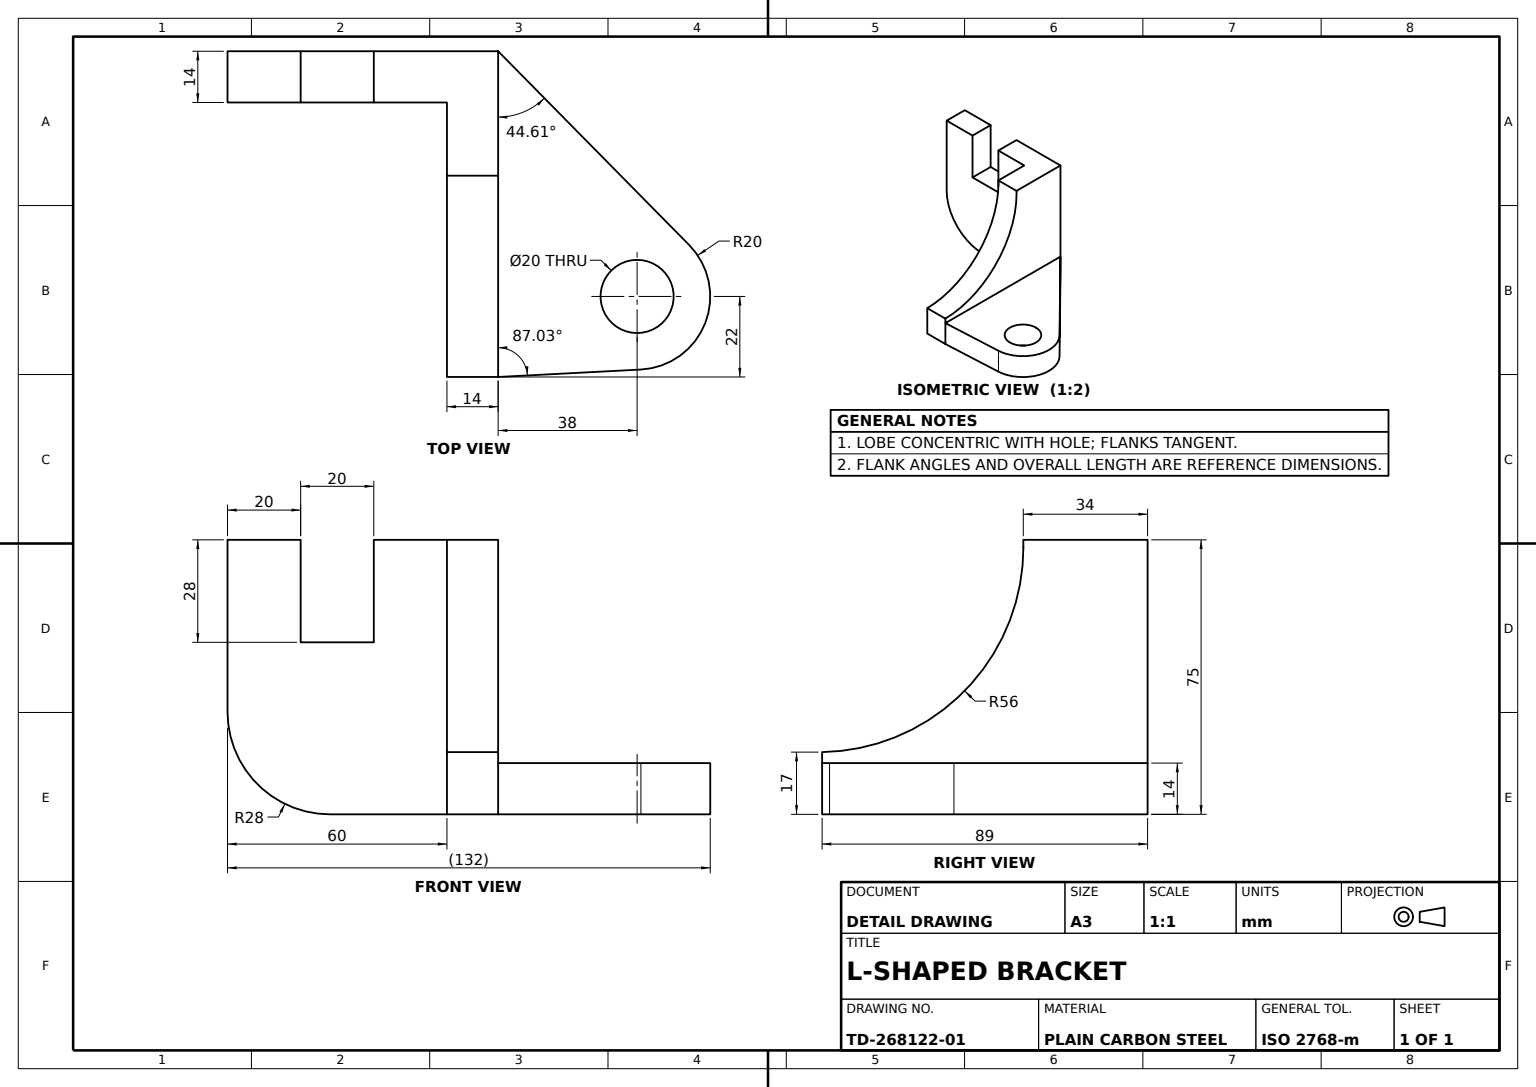
SolidWorks part; units mm, degrees
material "Plain Carbon Steel"
ref_plane "Front Plane" through (0, 0, 0) normal (0, 0, 1) x (1, 0, 0)
ref_plane "Top Plane" through (0, 0, 0) normal (0, 1, 0) x (1, 0, 0)
ref_plane "Right Plane" through (0, 0, 0) normal (1, 0, 0) x (0, 0, -1)
sketch "Base Plate Profile" plane through (0, 0, 0) normal (0, 0, 1) x (1, 0, 0)
  line L0 (0, 0) -> (0, 75)
  line L1 (0, 75) -> (32, 75)
  line L2 (60, 47) -> (60, 0)
  line L3 (60, 0) -> (40, 0)
  line L4 (40, 0) -> (40, 28)
  line L5 (40, 28) -> (20, 28)
  line L6 (20, 28) -> (20, 0)
  line L7 (20, 0) -> (0, 0)
  arc A0 (60, 47) -> (32, 75) centre (32, 47) ccw
  dimension "D6" = 28
  dimension "D1" = 75
  dimension "D2" = 20
  dimension "D3" = 20
  dimension "D4" = 60
  dimension "D5" = 28
extrude "Base Plate 14mm" add sketch "Base Plate Profile" along normal mid plane 14
sketch "Side Plate Profile" plane through (0, 0, 0) normal (-1, 0, 0) x (0, 0, 1)
  line L0 (-7, 75) -> (82, 75)
  line L1 (82, 75) -> (82, 58)
  line L2 (7, 0) -> (27, 0)
  line L7 (-7, 75) -> (-7, 0)
  line L8 (-7, 0) -> (7, 0)
  line L9 (7, 0) -> (7, 75)
  line L10 (7, 75) -> (-7, 75)
  line L11 (-7, 75) -> (-7, 0)
  line L12 (-7, 0) -> (7, 0)
  arc A0 (27, 0) -> (82, 58) centre (82.964, 2.0083) cw
  dimension "D4" = 56
  dimension "D1" = 89
  dimension "D2" = 20
  dimension "D3" = 17
  dimension "D5" = 0
extrude "Side Plate 14mm" add sketch "Side Plate Profile" along normal blind 14
sketch "Slotted End Plate Profile" plane through (0, 75, 0) normal (0, 1, 0) x (1, 0, 0)
  line L0 (-60.3344, -60) -> (-14, -60) construction
  line L2 (-52, -44.5) -> (-52, -87.389) construction
  line L3 (-52, -87.389) -> (-52, -9.5343) construction
  line L4 (-14, -82) -> (-14, 7) construction
  line L5 (-14, -82) -> (-53.0371, -79.9731)
  line L6 (-14, 7) -> (-66.2381, -45.9545)
  circle A0 centre (-52, -60) radius 10
  arc A1 (-66.2381, -45.9545) -> (-52, -80) centre (-52, -60) ccw
  dimension "D3" = 20
  dimension "D4" = 40
  dimension "D1" = 38
  dimension "D2" = 22
  dimension "D5" = 46.3344
  dimension "D6" = 27.389
extrude "Slotted End Plate 14mm" add sketch "Slotted End Plate Profile" against normal blind 14
